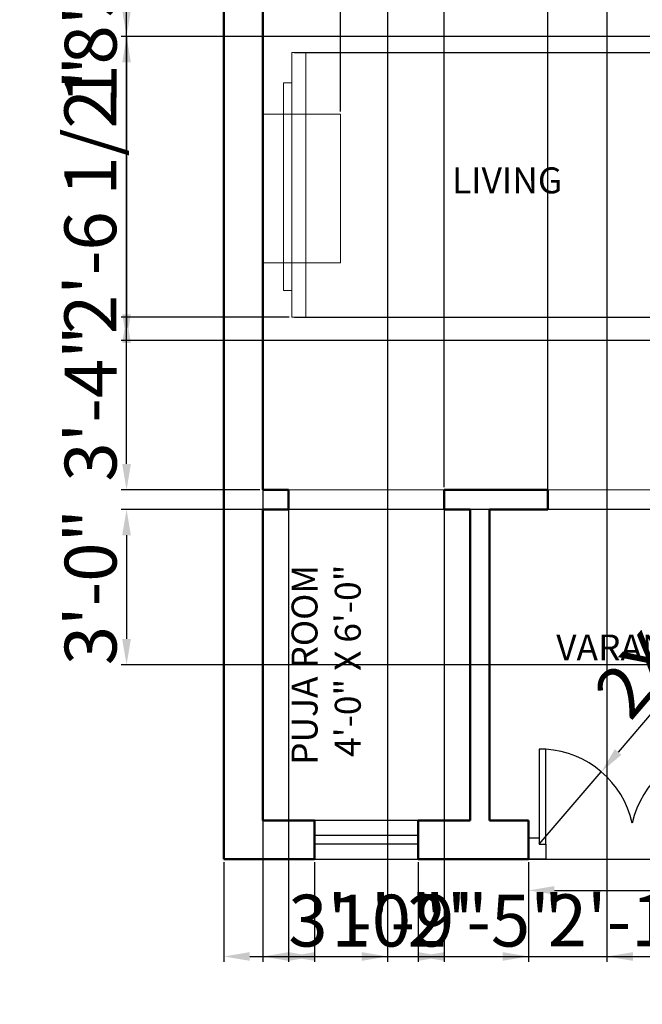
# Model space of a CAD drawing. Units: inches. Extents: x 1086 to 1501, y 383 to 973.
# Tile 1 of 7: x 1086 to 1230, y 383 to 611. Entities that reach past the tile are written whole.
import ezdxf

# ---------------------------------------------------------------- set-up
doc = ezdxf.new("R2010")
doc.units = ezdxf.units.IN
for name, color, linetype, lineweight in [('A-ANNO-DIMS', 2, 'Continuous', 18), ('A-AREA-IDEN', 7, 'Continuous', 25), ('A-EQPM', 8, 'Continuous', 18), ('door', 10, 'Continuous', 25), ('furniture', 255, 'Continuous', 18), ('opening', 219, 'Continuous', 18), ('ventilator', 151, 'Continuous', 25), ('wall', 7, 'Continuous', 50)]:
    doc.layers.add(name, color=color, linetype=linetype, lineweight=lineweight)
doc.styles.get("Standard").update_dxf_attribs({"font": 'arial.ttf'})
doc.dimstyles.new('ISO-25', dxfattribs={"dimtxt": 12, "dimasz": 6, "dimexe": 1.25, "dimexo": 0.625, "dimtad": 1, "dimdec": 1, "dimlunit": 3, "dimtxsty": 'Standard', "dimcen": 2.5, "dimadec": 0, "dimazin": 0, "dimtfac": 1, "dimtdec": 1, "dimtmove": 0, "dimatfit": 3, "dimfxl": 1, "dimarcsym": 0})

# ---------------------------------------------------------------- blocks, each defined once
blk = doc.blocks.new('d3')
at = {"layer": 'door'}
blk.add_line((1743.18, 564.73), (1791.18, 564.73), dxfattribs=at)
for points in [[(1745.68, 568.23), (1747.18, 568.23), (1747.18, 590.23), (1745.68, 590.23)], [(1787.18, 568.23), (1788.68, 568.23), (1788.68, 590.23), (1787.18, 590.23)]]:
    blk.add_lwpolyline(points, close=True, dxfattribs=at)
for points in [[(1747.18, 564.73), (1743.18, 564.73), (1743.18, 569.73), (1745.68, 569.73), (1745.68, 568.23), (1747.18, 568.23), (1747.18, 564.73)], [(1787.18, 564.73), (1791.18, 564.73), (1791.18, 569.73), (1788.68, 569.73), (1788.68, 568.23), (1787.18, 568.23), (1787.18, 564.73)]]:
    blk.add_lwpolyline(points, dxfattribs=at)
for centre, start, end in [((1745.68, 568.23), 12.8362, 86.0995), ((1788.68, 568.23), 93.9005, 167.1638)]:
    blk.add_arc(centre, 22.05, start, end, dxfattribs=at)
blk = doc.blocks.new('v')
at = {"layer": 'ventilator'}
for p, q in [((1539.56, 920.22), (1539.56, 896.22)), ((1541.56, 920.22), (1541.56, 896.22))]:
    blk.add_line(p, q, dxfattribs=at)
blk.add_lwpolyline([(1536.06, 896.22), (1545.06, 896.22), (1545.06, 920.22), (1536.06, 920.22)], close=True, dxfattribs=at)
blk = doc.blocks.new('*D21')
at = {"layer": 'A-ANNO-DIMS', "color": 0, "lineweight": -2, "transparency": 16777216}
for p, q in [((1203.93, 415.58), (1203.93, 407.76)), ((1251.93, 415.58), (1251.93, 407.76)), ((1209.93, 409.01), (1245.93, 409.01)), ((1251.93, 409.01), (1406.87, 409.01))]:
    blk.add_line(p, q, dxfattribs=at)
at = {"layer": 'A-ANNO-DIMS', "color": 0, "transparency": 16777216}
for points in [[(1209.93, 410.01), (1209.93, 408.01), (1203.93, 409.01)], [(1245.93, 410.01), (1245.93, 408.01), (1251.93, 409.01)]]:
    blk.add_solid(points, dxfattribs=at)
at = {"layer": 'Defpoints', "color": 0, "transparency": 16777216}
for p in [(1203.93, 416.21), (1251.93, 416.21), (1251.93, 409.01)]:
    blk.add_point(p, dxfattribs=at)
at = {"layer": 'A-ANNO-DIMS', "color": 0, "transparency": 16777216, "insert": (1332.4, 415.84), "char_height": 12, "attachment_point": 5}
blk.add_mtext('ENTRY DOOR 4\'-0"', dxfattribs=at)
blk = doc.blocks.new('*D38')
at = {"layer": 'A-ANNO-DIMS', "color": 0, "lineweight": -2, "transparency": 16777216}
for p, q in [((1133.43, 415.58), (1133.43, 392.46)), ((1154.43, 415.58), (1154.43, 392.46)), ((1139.43, 393.71), (1148.43, 393.71)), ((1154.43, 393.71), (1192.45, 393.71))]:
    blk.add_line(p, q, dxfattribs=at)
at = {"layer": 'A-ANNO-DIMS', "color": 0, "transparency": 16777216}
for points in [[(1139.43, 394.71), (1139.43, 392.71), (1133.43, 393.71)], [(1148.43, 394.71), (1148.43, 392.71), (1154.43, 393.71)]]:
    blk.add_solid(points, dxfattribs=at)
at = {"layer": 'Defpoints', "color": 0, "transparency": 16777216}
for p in [(1133.43, 416.21), (1154.43, 416.21), (1154.43, 393.71)]:
    blk.add_point(p, dxfattribs=at)
at = {"layer": 'A-ANNO-DIMS', "color": 0, "transparency": 16777216, "insert": (1176.44, 400.46), "char_height": 12, "attachment_point": 5}
blk.add_mtext('1\'-9"', dxfattribs=at)
blk = doc.blocks.new('*D39')
at = {"layer": 'A-ANNO-DIMS', "color": 0, "lineweight": -2, "transparency": 16777216}
for p, q in [((1178.43, 415.58), (1178.43, 392.46)), ((1203.93, 415.58), (1203.93, 392.46)), ((1184.43, 393.71), (1197.93, 393.71)), ((1203.93, 393.71), (1271.25, 393.71))]:
    blk.add_line(p, q, dxfattribs=at)
at = {"layer": 'A-ANNO-DIMS', "color": 0, "transparency": 16777216}
for points in [[(1184.43, 394.71), (1184.43, 392.71), (1178.43, 393.71)], [(1197.93, 394.71), (1197.93, 392.71), (1203.93, 393.71)]]:
    blk.add_solid(points, dxfattribs=at)
at = {"layer": 'Defpoints', "color": 0, "transparency": 16777216}
for p in [(1178.43, 416.21), (1203.93, 416.21), (1203.93, 393.71)]:
    blk.add_point(p, dxfattribs=at)
at = {"layer": 'A-ANNO-DIMS', "color": 0, "transparency": 16777216, "insert": (1240.59, 400.54), "char_height": 12, "attachment_point": 5}
blk.add_mtext('2\'-1 1/2"', dxfattribs=at)
blk = doc.blocks.new('*D40')
at = {"layer": 'A-ANNO-DIMS', "color": 0, "lineweight": -2, "transparency": 16777216}
for p, q in [((1142.43, 502.33), (1142.43, 867.19)), ((1269.93, 502.33), (1269.93, 867.19)), ((1148.43, 865.94), (1263.93, 865.94))]:
    blk.add_line(p, q, dxfattribs=at)
at = {"layer": 'A-ANNO-DIMS', "color": 0, "transparency": 16777216}
for points in [[(1148.43, 866.94), (1148.43, 864.94), (1142.43, 865.94)], [(1263.93, 866.94), (1263.93, 864.94), (1269.93, 865.94)]]:
    blk.add_solid(points, dxfattribs=at)
at = {"layer": 'Defpoints', "color": 0, "transparency": 16777216}
for p in [(1269.93, 865.94), (1142.43, 501.71), (1269.93, 501.71)]:
    blk.add_point(p, dxfattribs=at)
at = {"layer": 'A-ANNO-DIMS', "color": 0, "transparency": 16777216, "insert": (1206.18, 872.77), "char_height": 12, "attachment_point": 5}
blk.add_mtext('10\'-7 1/2"', dxfattribs=at)
blk = doc.blocks.new('*D41')
at = {"layer": 'A-ANNO-DIMS', "color": 0, "lineweight": -2, "transparency": 16777216}
for p, q in [((1141.8, 725.71), (1109.68, 725.71)), ((1110.93, 507.71), (1110.93, 719.71)), ((1141.8, 501.71), (1109.68, 501.71))]:
    blk.add_line(p, q, dxfattribs=at)
at = {"layer": 'A-ANNO-DIMS', "color": 0, "transparency": 16777216}
for points in [[(1109.93, 719.71), (1111.93, 719.71), (1110.93, 725.71)], [(1109.93, 507.71), (1111.93, 507.71), (1110.93, 501.71)]]:
    blk.add_solid(points, dxfattribs=at)
at = {"layer": 'Defpoints', "color": 0, "transparency": 16777216}
for p in [(1110.93, 725.71), (1142.43, 725.71), (1142.43, 501.71)]:
    blk.add_point(p, dxfattribs=at)
at = {"layer": 'A-ANNO-DIMS', "color": 0, "transparency": 16777216, "insert": (1104.18, 613.71), "char_height": 12, "attachment_point": 5, "rotation": 90}
blk.add_mtext('18\'-8"', dxfattribs=at)
blk = doc.blocks.new('*D43')
at = {"layer": 'A-ANNO-DIMS', "color": 0, "lineweight": -2, "transparency": 16777216}
for p, q in [((1208.43, 497.83), (1208.43, 867.19)), ((1256.43, 497.83), (1256.43, 867.19)), ((1214.43, 865.94), (1250.43, 865.94))]:
    blk.add_line(p, q, dxfattribs=at)
at = {"layer": 'A-ANNO-DIMS', "color": 0, "transparency": 16777216}
for points in [[(1214.43, 866.94), (1214.43, 864.94), (1208.43, 865.94)], [(1250.43, 866.94), (1250.43, 864.94), (1256.43, 865.94)]]:
    blk.add_solid(points, dxfattribs=at)
at = {"layer": 'Defpoints', "color": 0, "transparency": 16777216}
for p in [(1256.43, 865.94), (1208.43, 497.21), (1256.43, 497.21)]:
    blk.add_point(p, dxfattribs=at)
at = {"layer": 'A-ANNO-DIMS', "color": 0, "transparency": 16777216, "insert": (1232.43, 872.69), "char_height": 12, "attachment_point": 5}
blk.add_mtext('4\'-0"', dxfattribs=at)
blk = doc.blocks.new('*D44')
at = {"layer": 'A-ANNO-DIMS', "color": 0, "lineweight": -2, "transparency": 16777216}
for p, q in [((1258.8, 497.21), (1109.68, 497.21)), ((1110.93, 491.21), (1110.93, 467.21)), ((1258.8, 461.21), (1109.68, 461.21))]:
    blk.add_line(p, q, dxfattribs=at)
at = {"layer": 'A-ANNO-DIMS', "color": 0, "transparency": 16777216}
for points in [[(1109.93, 491.21), (1111.93, 491.21), (1110.93, 497.21)], [(1109.93, 467.21), (1111.93, 467.21), (1110.93, 461.21)]]:
    blk.add_solid(points, dxfattribs=at)
at = {"layer": 'Defpoints', "color": 0, "transparency": 16777216}
for p in [(1259.43, 497.21), (1110.93, 461.21), (1259.43, 461.21)]:
    blk.add_point(p, dxfattribs=at)
at = {"layer": 'A-ANNO-DIMS', "color": 0, "transparency": 16777216, "insert": (1104.17, 479.21), "char_height": 12, "attachment_point": 5, "rotation": 90}
blk.add_mtext('3\'-0"', dxfattribs=at)
blk = doc.blocks.new('*D50')
at = {"layer": 'A-ANNO-DIMS', "color": 0, "lineweight": -2, "transparency": 16777216}
for p, q in [((1184.43, 502.33), (1184.43, 867.19)), ((1208.43, 502.33), (1208.43, 867.19)), ((1190.43, 865.94), (1202.43, 865.94)), ((1208.43, 865.94), (1247.78, 865.94))]:
    blk.add_line(p, q, dxfattribs=at)
at = {"layer": 'A-ANNO-DIMS', "color": 0, "transparency": 16777216}
for points in [[(1190.43, 866.94), (1190.43, 864.94), (1184.43, 865.94)], [(1202.43, 866.94), (1202.43, 864.94), (1208.43, 865.94)]]:
    blk.add_solid(points, dxfattribs=at)
at = {"layer": 'Defpoints', "color": 0, "transparency": 16777216}
for p in [(1208.43, 865.94), (1184.43, 501.71), (1208.43, 501.71)]:
    blk.add_point(p, dxfattribs=at)
at = {"layer": 'A-ANNO-DIMS', "color": 0, "transparency": 16777216, "insert": (1231.11, 872.69), "char_height": 12, "attachment_point": 5}
blk.add_mtext('2\'-0"', dxfattribs=at)
blk = doc.blocks.new('*D51')
at = {"layer": 'A-ANNO-DIMS', "color": 0, "lineweight": -2, "transparency": 16777216}
for p, q in [((1148.43, 501.08), (1148.43, 392.46)), ((1184.43, 501.08), (1184.43, 392.46)), ((1154.43, 393.71), (1178.43, 393.71))]:
    blk.add_line(p, q, dxfattribs=at)
at = {"layer": 'A-ANNO-DIMS', "color": 0, "transparency": 16777216}
for points in [[(1154.43, 394.71), (1154.43, 392.71), (1148.43, 393.71)], [(1178.43, 394.71), (1178.43, 392.71), (1184.43, 393.71)]]:
    blk.add_solid(points, dxfattribs=at)
at = {"layer": 'Defpoints', "color": 0, "transparency": 16777216}
for p in [(1148.43, 501.71), (1184.43, 501.71), (1184.43, 393.71)]:
    blk.add_point(p, dxfattribs=at)
at = {"layer": 'A-ANNO-DIMS', "color": 0, "transparency": 16777216, "insert": (1166.43, 400.46), "char_height": 12, "attachment_point": 5}
blk.add_mtext('3\'-0"', dxfattribs=at)
blk = doc.blocks.new('*D58')
at = {"layer": 'A-ANNO-DIMS', "color": 0, "lineweight": -2, "transparency": 16777216}
for p, q in [((1250.08, 809.82), (1250.08, 392.46)), ((1222.08, 799.32), (1222.08, 392.46)), ((1228.08, 393.71), (1244.08, 393.71)), ((1250.08, 393.71), (1289.44, 393.71))]:
    blk.add_line(p, q, dxfattribs=at)
at = {"layer": 'A-ANNO-DIMS', "color": 0, "transparency": 16777216}
for points in [[(1228.08, 394.71), (1228.08, 392.71), (1222.08, 393.71)], [(1244.08, 394.71), (1244.08, 392.71), (1250.08, 393.71)]]:
    blk.add_solid(points, dxfattribs=at)
at = {"layer": 'Defpoints', "color": 0, "transparency": 16777216}
for p in [(1250.08, 810.44), (1222.08, 799.94), (1250.08, 393.71)]:
    blk.add_point(p, dxfattribs=at)
at = {"layer": 'A-ANNO-DIMS', "color": 0, "transparency": 16777216, "insert": (1272.76, 400.36), "char_height": 12, "attachment_point": 5}
blk.add_mtext('2\'-4"', dxfattribs=at)
blk = doc.blocks.new('*D63')
at = {"layer": 'A-ANNO-DIMS', "color": 0, "lineweight": -2, "transparency": 16777216}
for p, q in [((1142.43, 632.08), (1142.43, 392.46)), ((1171.32, 632.08), (1171.32, 392.46)), ((1148.43, 393.71), (1165.32, 393.71)), ((1171.32, 393.71), (1210.68, 393.71))]:
    blk.add_line(p, q, dxfattribs=at)
at = {"layer": 'A-ANNO-DIMS', "color": 0, "transparency": 16777216}
for points in [[(1148.43, 394.71), (1148.43, 392.71), (1142.43, 393.71)], [(1165.32, 394.71), (1165.32, 392.71), (1171.32, 393.71)]]:
    blk.add_solid(points, dxfattribs=at)
at = {"layer": 'Defpoints', "color": 0, "transparency": 16777216}
for p in [(1142.43, 632.71), (1171.32, 632.71), (1171.32, 393.71)]:
    blk.add_point(p, dxfattribs=at)
at = {"layer": 'A-ANNO-DIMS', "color": 0, "transparency": 16777216, "insert": (1194, 400.46), "char_height": 12, "attachment_point": 5}
blk.add_mtext('2\'-5"', dxfattribs=at)
blk = doc.blocks.new('*D68')
at = {"layer": 'A-ANNO-DIMS', "color": 0, "lineweight": -2, "transparency": 16777216}
for p, q in [((1110.93, 606.65), (1110.93, 683.08)), ((1262.93, 606.65), (1109.68, 606.65)), ((1110.93, 542.31), (1110.93, 600.65)), ((1262.93, 536.31), (1109.68, 536.31))]:
    blk.add_line(p, q, dxfattribs=at)
at = {"layer": 'A-ANNO-DIMS', "color": 0, "transparency": 16777216}
for points in [[(1109.93, 600.65), (1111.93, 600.65), (1110.93, 606.65)], [(1109.93, 542.31), (1111.93, 542.31), (1110.93, 536.31)]]:
    blk.add_solid(points, dxfattribs=at)
at = {"layer": 'Defpoints', "color": 0, "transparency": 16777216}
for p in [(1110.93, 606.65), (1263.55, 606.65), (1263.55, 536.31)]:
    blk.add_point(p, dxfattribs=at)
at = {"layer": 'A-ANNO-DIMS', "color": 0, "transparency": 16777216, "insert": (1104.1, 647.86), "char_height": 12, "attachment_point": 5, "rotation": 90}
blk.add_mtext('5\'-10 1/2"', dxfattribs=at)
blk = doc.blocks.new('*D70')
at = {"layer": 'A-ANNO-DIMS', "color": 0, "lineweight": -2, "transparency": 16777216}
for p, q in [((1269.3, 637.21), (1109.68, 637.21)), ((1110.93, 631.21), (1110.93, 612.65)), ((1262.93, 606.65), (1109.68, 606.65)), ((1110.93, 606.65), (1110.93, 539.33))]:
    blk.add_line(p, q, dxfattribs=at)
at = {"layer": 'A-ANNO-DIMS', "color": 0, "transparency": 16777216}
for points in [[(1109.93, 631.21), (1111.93, 631.21), (1110.93, 637.21)], [(1109.93, 612.65), (1111.93, 612.65), (1110.93, 606.65)]]:
    blk.add_solid(points, dxfattribs=at)
at = {"layer": 'Defpoints', "color": 0, "transparency": 16777216}
for p in [(1269.93, 637.21), (1110.93, 606.65), (1263.55, 606.65)]:
    blk.add_point(p, dxfattribs=at)
at = {"layer": 'A-ANNO-DIMS', "color": 0, "transparency": 16777216, "insert": (1104.1, 569.99), "char_height": 12, "attachment_point": 5, "rotation": 90}
blk.add_mtext('2\'-6 1/2"', dxfattribs=at)
blk = doc.blocks.new('*D71')
at = {"layer": 'A-ANNO-DIMS', "color": 0, "lineweight": -2, "transparency": 16777216}
for p, q in [((1142.43, 589.29), (1142.43, 867.19)), ((1160.43, 589.29), (1160.43, 867.19)), ((1148.43, 865.94), (1154.43, 865.94)), ((1160.43, 865.94), (1198.45, 865.94))]:
    blk.add_line(p, q, dxfattribs=at)
at = {"layer": 'A-ANNO-DIMS', "color": 0, "transparency": 16777216}
for points in [[(1148.43, 866.94), (1148.43, 864.94), (1142.43, 865.94)], [(1154.43, 866.94), (1154.43, 864.94), (1160.43, 865.94)]]:
    blk.add_solid(points, dxfattribs=at)
at = {"layer": 'Defpoints', "color": 0, "transparency": 16777216}
for p in [(1160.43, 865.94), (1142.43, 588.67), (1160.43, 588.67)]:
    blk.add_point(p, dxfattribs=at)
at = {"layer": 'A-ANNO-DIMS', "color": 0, "transparency": 16777216, "insert": (1182.44, 872.69), "char_height": 12, "attachment_point": 5}
blk.add_mtext('1\'-6"', dxfattribs=at)
blk = doc.blocks.new('*D72')
at = {"layer": 'A-ANNO-DIMS', "color": 0, "lineweight": -2, "transparency": 16777216}
for p, q in [((1149.81, 602.97), (1428.36, 602.97)), ((1427.11, 596.97), (1427.11, 547.72)), ((1149.81, 541.72), (1428.36, 541.72))]:
    blk.add_line(p, q, dxfattribs=at)
at = {"layer": 'A-ANNO-DIMS', "color": 0, "transparency": 16777216}
for points in [[(1426.11, 596.97), (1428.11, 596.97), (1427.11, 602.97)], [(1426.11, 547.72), (1428.11, 547.72), (1427.11, 541.72)]]:
    blk.add_solid(points, dxfattribs=at)
at = {"layer": 'Defpoints', "color": 0, "transparency": 16777216}
for p in [(1149.18, 602.97), (1149.18, 541.72), (1427.11, 541.72)]:
    blk.add_point(p, dxfattribs=at)
at = {"layer": 'A-ANNO-DIMS', "color": 0, "transparency": 16777216, "insert": (1420.36, 572.35), "char_height": 12, "attachment_point": 5, "rotation": 90}
blk.add_mtext('5\'-1"', dxfattribs=at)
blk = doc.blocks.new('*D73')
at = {"layer": 'A-ANNO-DIMS', "color": 0, "lineweight": -2, "transparency": 16777216}
for p, q in [((1148.56, 541.72), (1109.68, 541.72)), ((1110.93, 507.71), (1110.93, 535.72)), ((1141.8, 501.71), (1109.68, 501.71))]:
    blk.add_line(p, q, dxfattribs=at)
at = {"layer": 'A-ANNO-DIMS', "color": 0, "transparency": 16777216}
for points in [[(1109.93, 535.72), (1111.93, 535.72), (1110.93, 541.72)], [(1109.93, 507.71), (1111.93, 507.71), (1110.93, 501.71)]]:
    blk.add_solid(points, dxfattribs=at)
at = {"layer": 'Defpoints', "color": 0, "transparency": 16777216}
for p in [(1110.93, 541.72), (1149.18, 541.72), (1142.43, 501.71)]:
    blk.add_point(p, dxfattribs=at)
at = {"layer": 'A-ANNO-DIMS', "color": 0, "transparency": 16777216, "insert": (1104.17, 521.71), "char_height": 12, "attachment_point": 5, "rotation": 90}
blk.add_mtext('3\'-4"', dxfattribs=at)
blk = doc.blocks.new('*D80')
at = {"layer": 'A-ANNO-DIMS', "color": 0, "lineweight": -2, "transparency": 16777216}
for p, q in [((1280.51, 506.35), (1224.66, 441.03)), ((1206.43, 419.71), (1220.76, 436.47))]:
    blk.add_line(p, q, dxfattribs=at)
at = {"layer": 'A-ANNO-DIMS', "color": 0, "transparency": 16777216}
blk.add_solid([(1223.9, 441.68), (1225.42, 440.38), (1220.76, 436.47)], dxfattribs=at)
at = {"layer": 'Defpoints', "color": 0, "transparency": 16777216}
for p in [(1220.76, 436.47), (1206.43, 419.71)]:
    blk.add_point(p, dxfattribs=at)
at = {"layer": 'A-ANNO-DIMS', "color": 0, "transparency": 16777216, "insert": (1249.4, 480.36), "char_height": 12, "attachment_point": 5, "rotation": 49.4689}
blk.add_mtext('2X R1\'-10"', dxfattribs=at)

msp = doc.modelspace()

# ---------------------------------------------------------------- linework, layer by layer
at = {"layer": 'A-EQPM'}
for points in [[(1149.18, 602.97), (1152.41, 602.97), (1152.41, 541.72), (1149.18, 541.72)], [(1149.18, 595.91), (1147.26, 595.91), (1147.26, 547.83), (1149.18, 547.83)]]:
    msp.add_lwpolyline(points, close=True, dxfattribs=at)
at = {"layer": 'furniture'}
msp.add_lwpolyline([(1142.43, 588.67), (1160.43, 588.67), (1160.43, 554.29), (1142.43, 554.29)], close=True, dxfattribs=at)
at = {"layer": 'opening'}
for points in [[(1148.43, 501.71), (1184.43, 501.71), (1184.43, 497.21), (1148.43, 497.21)], [(1208.43, 501.71), (1256.43, 501.71), (1256.43, 497.21), (1208.43, 497.21)]]:
    msp.add_lwpolyline(points, close=True, dxfattribs=at)
at = {"layer": 'wall'}
for p, q in [((1133.43, 646.12), (1133.43, 416.21)), ((1142.43, 646.12), (1142.43, 501.71)), ((1142.43, 501.71), (1148.43, 501.71)), ((1148.43, 497.21), (1148.43, 501.71)), ((1184.43, 497.21), (1184.43, 501.71)), ((1184.43, 501.71), (1208.43, 501.71)), ((1208.43, 497.21), (1208.43, 501.71)), ((1142.43, 497.21), (1148.43, 497.21)), ((1142.43, 497.21), (1142.43, 425.21)), ((1184.43, 497.21), (1190.43, 497.21)), ((1190.43, 497.21), (1190.43, 425.21)), ((1194.93, 497.21), (1194.93, 425.21)), ((1194.93, 497.21), (1208.43, 497.21)), ((1142.43, 425.21), (1154.43, 425.21)), ((1154.43, 425.21), (1154.43, 416.21)), ((1178.43, 425.21), (1178.43, 416.21)), ((1178.43, 425.21), (1190.43, 425.21)), ((1194.93, 425.21), (1203.93, 425.21)), ((1203.93, 425.21), (1203.93, 416.21)), ((1133.43, 416.21), (1154.43, 416.21)), ((1178.43, 416.21), (1203.93, 416.21))]:
    msp.add_line(p, q, dxfattribs=at)

# ---------------------------------------------------------------- block references
at = {"layer": 'door'}
msp.add_blockref('d3', (-539.25, -148.53), dxfattribs=at)
at = {"layer": 'ventilator', "rotation": 270}
msp.add_blockref('v', (258.21, 1961.26), dxfattribs=at)

# ---------------------------------------------------------------- texts
at = {"layer": 'A-AREA-IDEN', "char_height": 6, "attachment_point": 1}
for s, insert in [(' LIVING', (1184.39, 576.36)), (' VARANDA', (1208.5, 468.24))]:
    msp.add_mtext_dynamic_manual_height_columns(s, width=53.2651, gutter_width=12.5, heights=[0], dxfattribs=dict(at, insert=insert))
at = {"layer": 'A-AREA-IDEN', "insert": (1149.11, 436.24), "char_height": 6, "attachment_point": 1, "rotation": 90}
msp.add_mtext_dynamic_manual_height_columns(' PUJA ROOM\\P  4\'-0" X 6\'-0"', width=53.2651, gutter_width=12.5, heights=[0], dxfattribs=at)

# ---------------------------------------------------------------- dimensions: what is measured, and where the dimension line sits
at = {"layer": 'A-ANNO-DIMS'}
for base, p1, p2, picture, middle in [((1269.93, 865.94), (1142.43, 501.71), (1269.93, 501.71), '*D40', (1206.18, 872.77)), ((1160.43, 865.94), (1142.43, 588.67), (1160.43, 588.67), '*D71', (1182.44, 872.69)), ((1208.43, 865.94), (1184.43, 501.71), (1208.43, 501.71), '*D50', (1231.11, 872.69)), ((1256.43, 865.94), (1208.43, 497.21), (1256.43, 497.21), '*D43', (1232.43, 872.69)), ((1250.08, 393.71), (1222.08, 799.94), (1250.08, 810.44), '*D58', (1272.76, 400.36)), ((1171.32, 393.71), (1142.43, 632.71), (1171.32, 632.71), '*D63', (1194, 400.46)), ((1184.43, 393.71), (1148.43, 501.71), (1184.43, 501.71), '*D51', (1166.43, 400.46)), ((1203.93, 393.71), (1178.43, 416.21), (1203.93, 416.21), '*D39', (1240.59, 400.54)), ((1154.43, 393.71), (1133.43, 416.21), (1154.43, 416.21), '*D38', (1176.44, 400.46))]:
    dim = msp.add_linear_dim(base=base, p1=p1, p2=p2, dimstyle='ISO-25', override={"dimdec": 1, "dimlfac": 1, "dimrnd": 0, "dimzin": 1, "dimdsep": 46, "dimlunit": 4, "dimfrac": 2}, dxfattribs=at)
    dim.commit()
    dim.dimension.update_dxf_attribs({"geometry": picture, "text_midpoint": middle})
for base, p1, p2, picture, middle in [((1110.93, 725.71), (1142.43, 501.71), (1142.43, 725.71), '*D41', (1104.18, 613.71)), ((1110.93, 606.65), (1263.55, 536.31), (1263.55, 606.65), '*D68', (1104.1, 647.86)), ((1110.93, 606.65), (1269.93, 637.21), (1263.55, 606.65), '*D70', (1104.1, 569.99)), ((1427.113, 541.7232), (1149.183, 602.9726), (1149.183, 541.7232), '*D72', (1420.3612, 572.3479)), ((1110.93, 541.72), (1142.43, 501.71), (1149.18, 541.72), '*D73', (1104.17, 521.71)), ((1110.93, 461.21), (1259.43, 497.21), (1259.43, 461.21), '*D44', (1104.17, 479.21))]:
    dim = msp.add_linear_dim(base=base, p1=p1, p2=p2, angle=90, dimstyle='ISO-25', override={"dimdec": 1, "dimlfac": 1, "dimrnd": 0, "dimzin": 1, "dimdsep": 46, "dimlunit": 4, "dimfrac": 2}, dxfattribs=at)
    dim.commit()
    dim.dimension.update_dxf_attribs({"geometry": picture, "text_midpoint": middle})
dim = msp.add_radius_dim(center=(1206.43, 419.71), mpoint=(1220.76, 436.47), text='2X <>', dimstyle='ISO-25', override={"dimdec": 1, "dimlfac": 1, "dimrnd": 0, "dimzin": 1, "dimdsep": 46, "dimlunit": 4, "dimfrac": 2}, dxfattribs=at)
dim.commit()
dim.dimension.update_dxf_attribs({"geometry": '*D80', "text_midpoint": (1249.4, 480.36)})
dim = msp.add_linear_dim(base=(1251.93, 409.01), p1=(1203.93, 416.21), p2=(1251.93, 416.21), text='ENTRY DOOR <>', dimstyle='ISO-25', override={"dimdec": 1, "dimlfac": 1, "dimrnd": 0, "dimzin": 1, "dimdsep": 46, "dimlunit": 4, "dimfrac": 2}, dxfattribs=at)
dim.commit()
dim.dimension.update_dxf_attribs({"geometry": '*D21', "text_midpoint": (1332.4, 415.84)})

doc.saveas('drawing.dxf')
